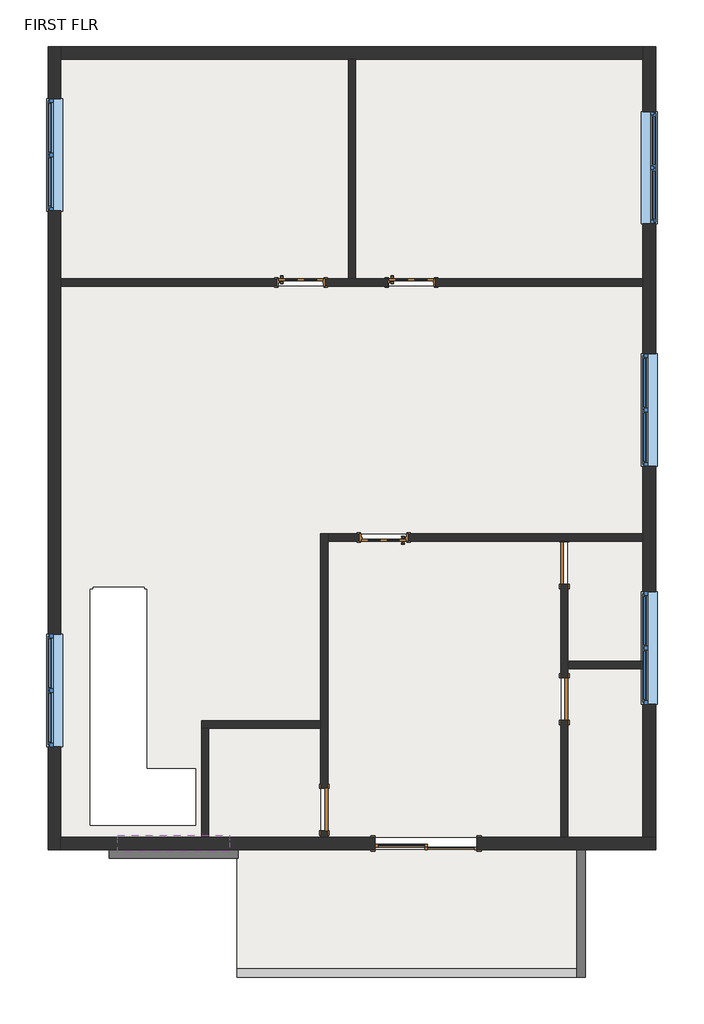
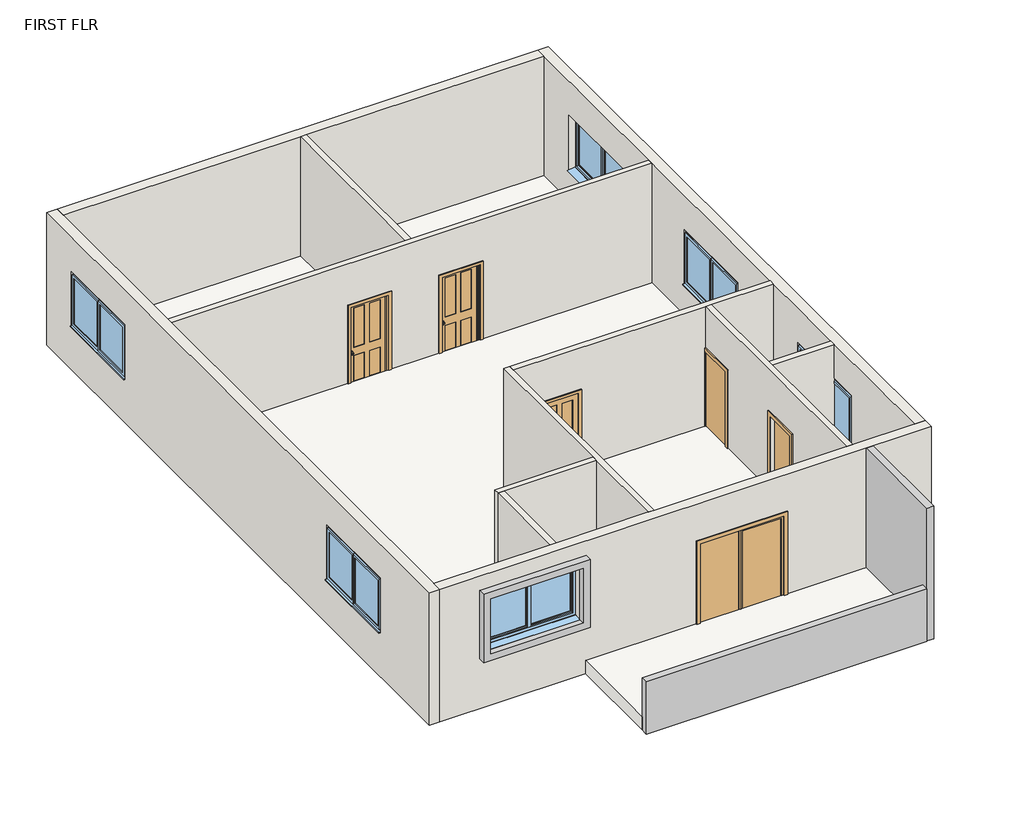
# One storey, incomplete: 12 walls, 7 doors, 6 windows, 3 proxies, 1 slab.
"""IFC4 building model written with IfcOpenShell, lengths in millimetres."""

from ifc_helpers import new_model, si_unit, frame, origin, place, context, project, spatial, polyline, outline, extrude, faceted_brep, transform, mapped, element, save
from components import generic_models_1_generic_models_1_b00c282c, generic_models_2_generic_models_2_90455f6d, generic_models_6_generic_models_6_ad273a16, door_d4d75d1e, door_interior_single_4_panel_wood_door_interior_single_4_d89ef9d3, door_1fe7f57d, door_e00f436c, w2_w2_7b90d420

model = new_model("IFC4")

# Units and contexts
model_context = context("Model", 3, world=origin())
ifc_project = project(units=[si_unit("LENGTHUNIT", "METRE", prefix="MILLI")], contexts=[model_context])

# Site, building, storey
site = spatial("IfcSite", under=ifc_project)
building = spatial("IfcBuilding", under=site)
storey = spatial("IfcBuildingStorey", under=building, Name="FIRST FLR", Elevation=3352.8)

# Proxies
placement = place(None, origin())
generic_models_1_generic_models_1_shape = generic_models_1_generic_models_1_b00c282c(model_context)
element("IfcBuildingElementProxy", 1, Name="Generic Models 1 : Generic Models 1", ObjectType="Generic Models 1 : Generic Models 1", at=placement, inside=storey, context=model_context, shape_type="MappedRepresentation", body=[
    mapped(generic_models_1_generic_models_1_shape, transform((0.0, 0.0, 0.0), x_axis=(1.0, 0.0, 0.0), y_axis=(0.0, 1.0, 0.0), z_axis=(0.0, 0.0, 1.0))),
])
generic_models_2_generic_models_2_shape = generic_models_2_generic_models_2_90455f6d(model_context)
element("IfcBuildingElementProxy", 2, Name="Generic Models 2 : Generic Models 2", ObjectType="Generic Models 2 : Generic Models 2", at=placement, inside=storey, context=model_context, shape_type="MappedRepresentation", body=[
    mapped(generic_models_2_generic_models_2_shape, transform((0.0, 0.0, 0.0), x_axis=(1.0, 0.0, 0.0), y_axis=(0.0, 1.0, 0.0), z_axis=(0.0, 0.0, 1.0))),
])
generic_models_6_generic_models_6_shape = generic_models_6_generic_models_6_ad273a16(model_context)
element("IfcBuildingElementProxy", 3, Name="Generic Models 6 : Generic Models 6", ObjectType="Generic Models 6 : Generic Models 6", at=placement, inside=storey, context=model_context, shape_type="MappedRepresentation", body=[
    mapped(generic_models_6_generic_models_6_shape, transform((0.0, 0.0, 0.0), x_axis=(1.0, 0.0, 0.0), y_axis=(0.0, 1.0, 0.0), z_axis=(0.0, 0.0, 1.0))),
])

# Doors
door_shape = door_d4d75d1e(model_context)
element("IfcDoor", 4, ObjectType="Door-Double-Sliding : 72\" x 84\"", at=placement, inside=storey, context=model_context, shape_type="MappedRepresentation", body=[
    mapped(door_shape, transform((24.4764037, -4030.9938352, 3352.8), x_axis=(-1.0, 0.0, 0.0), y_axis=(0.0, -1.0, 0.0), z_axis=(0.0, 0.0, 1.0))),
])
door_interior_single_4_panel_wood_door_interior_single_4_shape = door_interior_single_4_panel_wood_door_interior_single_4_d89ef9d3(model_context)
element("IfcDoor", 5, ObjectType="Door-Interior-Single-4_Panel-Wood : Door-Interior-Single-4_Panel-Wood", at=placement, inside=storey, context=model_context, shape_type="MappedRepresentation", body=[
    mapped(door_interior_single_4_panel_wood_door_interior_single_4_shape, transform((-241.5474631, 5903.5811648, 3352.8), x_axis=(1.0, 0.0, 0.0), y_axis=(0.0, 1.0, 0.0), z_axis=(0.0, 0.0, 1.0))),
])
element("IfcDoor", 6, ObjectType="Door-Interior-Single-4_Panel-Wood : Door-Interior-Single-4_Panel-Wood", at=placement, inside=storey, context=model_context, shape_type="MappedRepresentation", body=[
    mapped(door_interior_single_4_panel_wood_door_interior_single_4_shape, transform((-2222.7474631, 5903.5811648, 3352.8), x_axis=(1.0, 0.0, 0.0), y_axis=(0.0, 1.0, 0.0), z_axis=(0.0, 0.0, 1.0))),
])
element("IfcDoor", 7, ObjectType="Door-Interior-Single-4_Panel-Wood : Door-Interior-Single-4_Panel-Wood", at=placement, inside=storey, context=model_context, shape_type="MappedRepresentation", body=[
    mapped(door_interior_single_4_panel_wood_door_interior_single_4_shape, transform((-737.5235963, 1325.2311648, 3352.8), x_axis=(-1.0, 0.0, 0.0), y_axis=(0.0, -1.0, 0.0), z_axis=(0.0, 0.0, 1.0))),
])
door_2_shape = door_1fe7f57d(model_context)
element("IfcDoor", 8, ObjectType="Single-Flush : 30\" x 80\"", at=placement, inside=storey, context=model_context, shape_type="MappedRepresentation", body=[
    mapped(door_2_shape, transform((2501.6525369, 871.2061648, 3352.8), x_axis=(0.0, 1.0, 0.0), y_axis=(-1.0, 0.0, 0.0), z_axis=(0.0, 0.0, 1.0))),
])
element("IfcDoor", 9, ObjectType="Single-Flush : 30\" x 80\"", at=placement, inside=storey, context=model_context, shape_type="MappedRepresentation", body=[
    mapped(door_2_shape, transform((2501.6525369, -1567.1938352, 3352.8), x_axis=(0.0, -1.0, 0.0), y_axis=(1.0, 0.0, 0.0), z_axis=(0.0, 0.0, 1.0))),
])
door_3_shape = door_e00f436c(model_context)
element("IfcDoor", 10, ObjectType="Single-Flush : 30\" x 80\"", at=placement, inside=storey, context=model_context, shape_type="MappedRepresentation", body=[
    mapped(door_3_shape, transform((-1804.3235963, -3548.3938352, 3352.8), x_axis=(0.0, 1.0, 0.0), y_axis=(-1.0, 0.0, 0.0), z_axis=(0.0, 0.0, 1.0))),
])

# Slab
element("IfcSlab", 11, ObjectType="MARBLE FLOORING 1'", at=placement, inside=storey, context=model_context, shape_type="SweptSolid", body=[
    extrude(outline(polyline([(-1371.8474631, 9900.9061648), (-1371.8474631, 5963.9061648), (-6528.0474631, 5963.9061648), (-6528.0474631, 9900.9061648), (-1371.8474631, 9900.9061648)])), frame((0.0, 0.0, 3352.8), z_axis=(0.0, 0.0, 1.0), x_axis=(1.0, 0.0, 0.0)), (0.0, 0.0, 1.0), 304.8),
    extrude(outline(polyline([(3911.3525369, 9900.9061648), (3911.3525369, 5963.9061648), (-1244.8474631, 5963.9061648), (-1244.8474631, 9900.9061648), (3911.3525369, 9900.9061648)])), frame((0.0, 0.0, 3352.8), z_axis=(0.0, 0.0, 1.0), x_axis=(1.0, 0.0, 0.0)), (0.0, 0.0, 1.0), 304.8),
    extrude(outline(polyline([(-1867.8235963, -2087.8938352), (-1867.8235963, -4043.6938352), (-3874.4235963, -4043.6938352), (-3874.4235963, -2087.8938352), (-1867.8235963, -2087.8938352)])), frame((0.0, 0.0, 3352.8), z_axis=(0.0, 0.0, 1.0), x_axis=(1.0, 0.0, 0.0)), (0.0, 0.0, 1.0), 304.8),
    extrude(outline(polyline([(3911.3525369, 1264.9061648), (3911.3525369, -894.0938352), (2565.1525369, -894.0938352), (2565.1525369, 1264.9061648), (3911.3525369, 1264.9061648)])), frame((0.0, 0.0, 3352.8), z_axis=(0.0, 0.0, 1.0), x_axis=(1.0, 0.0, 0.0)), (0.0, 0.0, 1.0), 304.8),
    extrude(outline(polyline([(3912.9151699, -1021.0938352), (3912.9151699, -4043.6938352), (2565.1525369, -4043.6938352), (2565.1525369, -1021.0938352), (3912.9151699, -1021.0938352)])), frame((0.0, 0.0, 3352.8), z_axis=(0.0, 0.0, 1.0), x_axis=(1.0, 0.0, 0.0)), (0.0, 0.0, 1.0), 304.8),
    extrude(outline(polyline([(2438.1525369, 1264.9061648), (2438.1525369, -4043.6938352), (-1740.8235963, -4043.6938352), (-1740.8235963, 1264.9061648), (2438.1525369, 1264.9061648)])), frame((0.0, 0.0, 3352.8), z_axis=(0.0, 0.0, 1.0), x_axis=(1.0, 0.0, 0.0)), (0.0, 0.0, 1.0), 304.8),
    extrude(outline(polyline([(-4001.4235963, -4043.6938352), (-6528.0474631, -4043.6938352), (-6528.0474631, 5836.9061648), (3911.3525369, 5836.9061648), (3911.3525369, 1391.9061648), (-1867.8235963, 1391.9061648), (-1867.8235963, -1960.8938352), (-4001.4235963, -1960.8938352), (-4001.4235963, -4043.6938352)]), holes=[polyline([(-4986.3750936, -2818.257314), (-4986.3750936, 402.8727516), (-5037.1750936, 402.8727516), (-5037.1750936, 434.6227516), (-5951.5750936, 434.6227516), (-5951.5750936, 402.8727516), (-6002.3750936, 402.8727516), (-6002.3750936, -3834.257314), (-4109.8601025, -3834.257314), (-4109.8601025, -2818.257314), (-4986.3750936, -2818.257314)])]), frame((0.0, 0.0, 3352.8), z_axis=(0.0, 0.0, 1.0), x_axis=(1.0, 0.0, 0.0)), (0.0, 0.0, 1.0), 304.8),
    extrude(outline(polyline([(2729.4546869, -4272.2938352), (2729.4546869, -6405.8938352), (-3366.5453131, -6405.8938352), (-3366.5453131, -4272.2938352), (2729.4546869, -4272.2938352)])), frame((0.0, 0.0, 3352.8), z_axis=(0.0, 0.0, 1.0), x_axis=(1.0, 0.0, 0.0)), (0.0, 0.0, 1.0), 304.8),
])

# Walls
element("IfcWall", 12, ObjectType="EXTERIOR WALL 9\"", at=placement, inside=storey, context=model_context, shape_type="Brep", body=[
    faceted_brep([(-6756.6474631, 10129.5061648, 3352.8), (-6756.6474631, -4272.2938352, 3352.8), (-6756.6474631, -4272.2938352, 6400.8), (-6756.6474631, 10129.5061648, 6400.8), (-6756.6474631, -409.7938352, 4352.8), (-6756.6474631, -409.7938352, 5612.8), (-6756.6474631, -2419.7938352, 5612.8), (-6756.6474631, -2419.7938352, 4352.8), (-6756.6474631, 9191.4061648, 4352.8), (-6756.6474631, 9191.4061648, 5612.8), (-6756.6474631, 7181.4061648, 5612.8), (-6756.6474631, 7181.4061648, 4352.8), (-6528.0474631, 10129.5061648, 3352.8), (-6528.0474631, 10129.5061648, 6400.8), (-6528.0474631, 9900.9061648, 6400.8), (-6528.0474631, 5963.9061648, 6400.8), (-6528.0474631, 5836.9061648, 6400.8), (-6528.0474631, -4043.6938352, 6400.8), (-6528.0474631, -4272.2938352, 6400.8), (-6528.0474631, -4272.2938352, 3352.8), (-6528.0474631, -4043.6938352, 3352.8), (-6528.0474631, 5836.9061648, 3352.8), (-6528.0474631, 5963.9061648, 3352.8), (-6528.0474631, 9900.9061648, 3352.8), (-6528.0474631, -409.7938352, 4352.8), (-6528.0474631, -2419.7938352, 4352.8), (-6528.0474631, -2419.7938352, 5612.8), (-6528.0474631, -409.7938352, 5612.8), (-6528.0474631, 9191.4061648, 4352.8), (-6528.0474631, 7181.4061648, 4352.8), (-6528.0474631, 7181.4061648, 5612.8), (-6528.0474631, 9191.4061648, 5612.8)], [[[0, 1, 2, 3], [4, 5, 6, 7], [8, 9, 10, 11]], [[12, 13, 14, 15, 16, 17, 18, 19, 20, 21, 22, 23], [24, 25, 26, 27], [28, 29, 30, 31]], [[1, 0, 12, 23, 22, 21, 20, 19]], [[3, 2, 18, 17, 16, 15, 14, 13]], [[2, 1, 19, 18]], [[0, 3, 13, 12]], [[5, 4, 24, 27]], [[6, 5, 27, 26]], [[7, 6, 26, 25]], [[4, 7, 25, 24]], [[9, 8, 28, 31]], [[10, 9, 31, 30]], [[11, 10, 30, 29]], [[8, 11, 29, 28]]]),
])
element("IfcWall", 13, ObjectType="EXTERIOR WALL 9\"", at=placement, inside=storey, context=model_context, shape_type="Brep", body=[
    faceted_brep([(-6528.0474631, -4272.2938352, 3352.8), (-889.9235963, -4272.2938352, 3352.8), (-889.9235963, -4272.2938352, 5486.4), (938.8764037, -4272.2938352, 5486.4), (938.8764037, -4272.2938352, 3352.8), (4139.9525369, -4272.2938352, 3352.8), (4139.9525369, -4272.2938352, 6400.8), (-6528.0474631, -4272.2938352, 6400.8), (-3503.7474631, -4272.2938352, 4657.6), (-5513.7474631, -4272.2938352, 4657.6), (-5513.7474631, -4272.2938352, 5917.6), (-3503.7474631, -4272.2938352, 5917.6), (-889.9235963, -4043.6938352, 5486.4), (-889.9235963, -4043.6938352, 3352.8), (-1740.8235963, -4043.6938352, 3352.8), (-1867.8235963, -4043.6938352, 3352.8), (-3874.4235963, -4043.6938352, 3352.8), (-4001.4235963, -4043.6938352, 3352.8), (-6528.0474631, -4043.6938352, 3352.8), (-6528.0474631, -4043.6938352, 6400.8), (-4001.4235963, -4043.6938352, 6400.8), (-3874.4235963, -4043.6938352, 6400.8), (-1867.8235963, -4043.6938352, 6400.8), (-1740.8235963, -4043.6938352, 6400.8), (2438.1525369, -4043.6938352, 6400.8), (2565.1525369, -4043.6938352, 6400.8), (3911.3525369, -4043.6938352, 6400.8), (4139.9525369, -4043.6938352, 6400.8), (4139.9525369, -4043.6938352, 3352.8), (3911.3525369, -4043.6938352, 3352.8), (2565.1525369, -4043.6938352, 3352.8), (2438.1525369, -4043.6938352, 3352.8), (938.8764037, -4043.6938352, 3352.8), (938.8764037, -4043.6938352, 5486.4), (-3503.7474631, -4043.6938352, 4657.6), (-3503.7474631, -4043.6938352, 5917.6), (-5513.7474631, -4043.6938352, 5917.6), (-5513.7474631, -4043.6938352, 4657.6)], [[[0, 1, 2, 3, 4, 5, 6, 7], [8, 9, 10, 11]], [[12, 13, 14, 15, 16, 17, 18, 19, 20, 21, 22, 23, 24, 25, 26, 27, 28, 29, 30, 31, 32, 33], [34, 35, 36, 37]], [[18, 17, 16, 15, 14, 13, 1, 0]], [[32, 31, 30, 29, 28, 5, 4]], [[7, 6, 27, 26, 25, 24, 23, 22, 21, 20, 19]], [[0, 7, 19, 18]], [[6, 5, 28, 27]], [[35, 34, 8, 11]], [[36, 35, 11, 10]], [[37, 36, 10, 9]], [[34, 37, 9, 8]], [[4, 3, 33, 32]], [[2, 1, 13, 12]], [[3, 2, 12, 33]]]),
])
element("IfcWall", 14, ObjectType="EXTERIOR WALL 9\"", at=placement, inside=storey, context=model_context, shape_type="Brep", body=[
    faceted_brep([(4139.9525369, -4043.6938352, 3352.8), (4139.9525369, 10129.5061648, 3352.8), (4139.9525369, 10129.5061648, 6400.8), (4139.9525369, -4043.6938352, 6400.8), (4139.9525369, 4619.4061648, 4352.8), (4139.9525369, 2609.4061648, 4352.8), (4139.9525369, 2609.4061648, 5612.8), (4139.9525369, 4619.4061648, 5612.8), (4139.9525369, 352.2061648, 4352.8), (4139.9525369, -1657.7938352, 4352.8), (4139.9525369, -1657.7938352, 5612.8), (4139.9525369, 352.2061648, 5612.8), (4139.9525369, 6952.8061648, 4352.8), (4139.9525369, 6952.8061648, 5612.8), (4139.9525369, 8962.8061648, 5612.8), (4139.9525369, 8962.8061648, 4352.8), (3911.3525369, -4043.6938352, 3352.8), (3911.3525369, -4043.6938352, 6400.8), (3911.3525369, -1021.0938352, 6400.8), (3911.3525369, -894.0938352, 6400.8), (3911.3525369, 5836.9061648, 6400.8), (3911.3525369, 5963.9061648, 6400.8), (3911.3525369, 9900.9061648, 6400.8), (3911.3525369, 10129.5061648, 6400.8), (3911.3525369, 10129.5061648, 3352.8), (3911.3525369, 9900.9061648, 3352.8), (3911.3525369, 5963.9061648, 3352.8), (3911.3525369, 5836.9061648, 3352.8), (3911.3525369, -894.0938352, 3352.8), (3911.3525369, -1021.0938352, 3352.8), (3911.3525369, 4619.4061648, 4352.8), (3911.3525369, 4619.4061648, 5612.8), (3911.3525369, 2609.4061648, 5612.8), (3911.3525369, 2609.4061648, 4352.8), (3911.3525369, 352.2061648, 4352.8), (3911.3525369, 352.2061648, 5612.8), (3911.3525369, -1657.7938352, 5612.8), (3911.3525369, -1657.7938352, 4352.8), (3911.3525369, 6952.8061648, 4352.8), (3911.3525369, 8962.8061648, 4352.8), (3911.3525369, 8962.8061648, 5612.8), (3911.3525369, 6952.8061648, 5612.8)], [[[0, 1, 2, 3], [4, 5, 6, 7], [8, 9, 10, 11], [12, 13, 14, 15]], [[16, 17, 18, 19, 20, 21, 22, 23, 24, 25, 26, 27, 28, 29], [30, 31, 32, 33], [34, 35, 36, 37], [38, 39, 40, 41]], [[1, 0, 16, 29, 28, 27, 26, 25, 24]], [[3, 2, 23, 22, 21, 20, 19, 18, 17]], [[0, 3, 17, 16]], [[2, 1, 24, 23]], [[31, 30, 4, 7]], [[32, 31, 7, 6]], [[33, 32, 6, 5]], [[30, 33, 5, 4]], [[35, 34, 8, 11]], [[36, 35, 11, 10]], [[37, 36, 10, 9]], [[34, 37, 9, 8]], [[13, 12, 38, 41]], [[14, 13, 41, 40]], [[15, 14, 40, 39]], [[12, 15, 39, 38]]]),
])
element("IfcWall", 15, ObjectType="EXTERIOR WALL 9\"", at=placement, inside=storey, context=model_context, shape_type="Brep", body=[
    faceted_brep([(3911.3525369, 10129.5061648, 3352.8), (-6528.0474631, 10129.5061648, 3352.8), (-6528.0474631, 10129.5061648, 6400.8), (3911.3525369, 10129.5061648, 6400.8), (3911.3525369, 9900.9061648, 3352.8), (3911.3525369, 9900.9061648, 6400.8), (-1244.8474631, 9900.9061648, 6400.8), (-1371.8474631, 9900.9061648, 6400.8), (-6528.0474631, 9900.9061648, 6400.8), (-6528.0474631, 9900.9061648, 3352.8), (-1371.8474631, 9900.9061648, 3352.8), (-1244.8474631, 9900.9061648, 3352.8)], [[[0, 1, 2, 3]], [[4, 5, 6, 7, 8, 9, 10, 11]], [[1, 0, 4, 11, 10, 9]], [[3, 2, 8, 7, 6, 5]], [[0, 3, 5, 4]], [[2, 1, 9, 8]]]),
])
element("IfcWall", 16, ObjectType="INTERIOR WALL 5\"", at=placement, inside=storey, context=model_context, shape_type="SweptSolid", body=[
    extrude(outline(polyline([(-1371.8474631, 5963.9061648), (-1371.8474631, 9900.9061648), (-1244.8474631, 9900.9061648), (-1244.8474631, 5963.9061648), (-1371.8474631, 5963.9061648)])), frame((0.0, 0.0, 3352.8), z_axis=(0.0, 0.0, 1.0), x_axis=(1.0, 0.0, 0.0)), (0.0, 0.0, 1.0), 3048.0),
])
element("IfcWall", 17, ObjectType="INTERIOR WALL 5\"", at=placement, inside=storey, context=model_context, shape_type="Brep", body=[
    faceted_brep([(3911.3525369, 5836.9061648, 6400.8), (-6528.0474631, 5836.9061648, 6400.8), (-6528.0474631, 5836.9061648, 3352.8), (-2654.5474631, 5836.9061648, 3352.8), (-2654.5474631, 5836.9061648, 5410.2), (-1790.9474631, 5836.9061648, 5410.2), (-1790.9474631, 5836.9061648, 3352.8), (-673.3474631, 5836.9061648, 3352.8), (-673.3474631, 5836.9061648, 5410.2), (190.2525369, 5836.9061648, 5410.2), (190.2525369, 5836.9061648, 3352.8), (3911.3525369, 5836.9061648, 3352.8), (-6528.0474631, 5963.9061648, 6400.8), (-1371.8474631, 5963.9061648, 6400.8), (-1244.8474631, 5963.9061648, 6400.8), (3911.3525369, 5963.9061648, 6400.8), (3911.3525369, 5963.9061648, 3352.8), (190.2525369, 5963.9061648, 3352.8), (190.2525369, 5963.9061648, 5410.2), (-673.3474631, 5963.9061648, 5410.2), (-673.3474631, 5963.9061648, 3352.8), (-1244.8474631, 5963.9061648, 3352.8), (-1371.8474631, 5963.9061648, 3352.8), (-1790.9474631, 5963.9061648, 3352.8), (-1790.9474631, 5963.9061648, 5410.2), (-2654.5474631, 5963.9061648, 5410.2), (-2654.5474631, 5963.9061648, 3352.8), (-6528.0474631, 5963.9061648, 3352.8)], [[[0, 1, 2, 3, 4, 5, 6, 7, 8, 9, 10, 11]], [[12, 13, 14, 15, 16, 17, 18, 19, 20, 21, 22, 23, 24, 25, 26, 27]], [[16, 11, 10, 17]], [[2, 27, 26, 3]], [[20, 7, 6, 23, 22, 21]], [[1, 0, 15, 14, 13, 12]], [[0, 11, 16, 15]], [[2, 1, 12, 27]], [[9, 18, 17, 10]], [[18, 9, 8, 19]], [[19, 8, 7, 20]], [[5, 24, 23, 6]], [[24, 5, 4, 25]], [[25, 4, 3, 26]]]),
])
element("IfcWall", 18, ObjectType="INTERIOR WALL 5\"", at=placement, inside=storey, context=model_context, shape_type="Brep", body=[
    faceted_brep([(-1867.8235963, 1391.9061648, 3352.8), (-1867.8235963, -1960.8938352, 3352.8), (-1867.8235963, -2087.8938352, 3352.8), (-1867.8235963, -3167.3938352, 3352.8), (-1867.8235963, -3167.3938352, 5384.8), (-1867.8235963, -3929.3938352, 5384.8), (-1867.8235963, -3929.3938352, 3352.8), (-1867.8235963, -4043.6938352, 3352.8), (-1867.8235963, -4043.6938352, 6400.8), (-1867.8235963, -2087.8938352, 6400.8), (-1867.8235963, -1960.8938352, 6400.8), (-1867.8235963, 1391.9061648, 6400.8), (-1740.8235963, -3167.3938352, 5384.8), (-1740.8235963, -3167.3938352, 3352.8), (-1740.8235963, 1264.9061648, 3352.8), (-1740.8235963, 1391.9061648, 3352.8), (-1740.8235963, 1391.9061648, 6400.8), (-1740.8235963, 1264.9061648, 6400.8), (-1740.8235963, -4043.6938352, 6400.8), (-1740.8235963, -4043.6938352, 3352.8), (-1740.8235963, -3929.3938352, 3352.8), (-1740.8235963, -3929.3938352, 5384.8)], [[[0, 1, 2, 3, 4, 5, 6, 7, 8, 9, 10, 11]], [[12, 13, 14, 15, 16, 17, 18, 19, 20, 21]], [[20, 19, 7, 6]], [[15, 14, 13, 3, 2, 1, 0]], [[11, 10, 9, 8, 18, 17, 16]], [[8, 7, 19, 18]], [[0, 11, 16, 15]], [[4, 3, 13, 12]], [[5, 4, 12, 21]], [[6, 5, 21, 20]]]),
])
element("IfcWall", 19, ObjectType="INTERIOR WALL 5\"", at=placement, inside=storey, context=model_context, shape_type="Brep", body=[
    faceted_brep([(-4001.4235963, -2087.8938352, 3352.8), (-3874.4235963, -2087.8938352, 3352.8), (-1867.8235963, -2087.8938352, 3352.8), (-1867.8235963, -2087.8938352, 6400.8), (-3874.4235963, -2087.8938352, 6400.8), (-4001.4235963, -2087.8938352, 6400.8), (-4001.4235963, -1960.8938352, 3352.8), (-4001.4235963, -1960.8938352, 6400.8), (-1867.8235963, -1960.8938352, 6400.8), (-1867.8235963, -1960.8938352, 3352.8)], [[[0, 1, 2, 3, 4, 5]], [[6, 7, 8, 9]], [[2, 1, 0, 6, 9]], [[5, 4, 3, 8, 7]], [[0, 5, 7, 6]], [[3, 2, 9, 8]]]),
])
element("IfcWall", 20, ObjectType="INTERIOR WALL 5\"", at=placement, inside=storey, context=model_context, shape_type="SweptSolid", body=[
    extrude(outline(polyline([(-3874.4235963, -2087.8938352), (-3874.4235963, -4043.6938352), (-4001.4235963, -4043.6938352), (-4001.4235963, -2087.8938352), (-3874.4235963, -2087.8938352)])), frame((0.0, 0.0, 3352.8), z_axis=(0.0, 0.0, 1.0), x_axis=(1.0, 0.0, 0.0)), (0.0, 0.0, 1.0), 3048.0),
])
element("IfcWall", 21, ObjectType="INTERIOR WALL 5\"", at=placement, inside=storey, context=model_context, shape_type="Brep", body=[
    faceted_brep([(3910.6764037, 1264.9061648, 3352.8), (3910.6764037, 1264.9061648, 6400.8), (2565.1525369, 1264.9061648, 6400.8), (2438.1525369, 1264.9061648, 6400.8), (-1740.8235963, 1264.9061648, 6400.8), (-1740.8235963, 1264.9061648, 3352.8), (-1169.3235963, 1264.9061648, 3352.8), (-1169.3235963, 1264.9061648, 5410.2), (-305.7235963, 1264.9061648, 5410.2), (-305.7235963, 1264.9061648, 3352.8), (2438.1525369, 1264.9061648, 3352.8), (2565.1525369, 1264.9061648, 3352.8), (3910.6764037, 1391.9061648, 6400.8), (3910.6764037, 1391.9061648, 3352.8), (-305.7235963, 1391.9061648, 3352.8), (-305.7235963, 1391.9061648, 5410.2), (-1169.3235963, 1391.9061648, 5410.2), (-1169.3235963, 1391.9061648, 3352.8), (-1740.8235963, 1391.9061648, 3352.8), (-1740.8235963, 1391.9061648, 6400.8)], [[[0, 1, 2, 3, 4, 5, 6, 7, 8, 9, 10, 11]], [[12, 13, 14, 15, 16, 17, 18, 19]], [[13, 0, 11, 10, 9, 14]], [[5, 18, 17, 6]], [[1, 0, 13, 12]], [[4, 3, 2, 1, 12, 19]], [[5, 4, 19, 18]], [[16, 7, 6, 17]], [[7, 16, 15, 8]], [[8, 15, 14, 9]]]),
])
element("IfcWall", 22, ObjectType="INTERIOR WALL 5\"", at=placement, inside=storey, context=model_context, shape_type="Brep", body=[
    faceted_brep([(2438.1525369, -1948.1938352, 5384.8), (2438.1525369, -1948.1938352, 3352.8), (2438.1525369, -4043.6938352, 3352.8), (2438.1525369, -4043.6938352, 6400.8), (2438.1525369, 1264.9061648, 6400.8), (2438.1525369, 1264.9061648, 3352.8), (2438.1525369, 1252.2061648, 3352.8), (2438.1525369, 1252.2061648, 5384.8), (2438.1525369, 490.2061648, 5384.8), (2438.1525369, 490.2061648, 3352.8), (2438.1525369, -1186.1938352, 3352.8), (2438.1525369, -1186.1938352, 5384.8), (2565.1525369, -4043.6938352, 3352.8), (2565.1525369, -1948.1938352, 3352.8), (2565.1525369, -1948.1938352, 5384.8), (2565.1525369, -1186.1938352, 5384.8), (2565.1525369, -1186.1938352, 3352.8), (2565.1525369, -1021.0938352, 3352.8), (2565.1525369, -894.0938352, 3352.8), (2565.1525369, 490.2061648, 3352.8), (2565.1525369, 490.2061648, 5384.8), (2565.1525369, 1252.2061648, 5384.8), (2565.1525369, 1252.2061648, 3352.8), (2565.1525369, 1264.9061648, 3352.8), (2565.1525369, 1264.9061648, 6400.8), (2565.1525369, -894.0938352, 6400.8), (2565.1525369, -1021.0938352, 6400.8), (2565.1525369, -4043.6938352, 6400.8)], [[[0, 1, 2, 3, 4, 5, 6, 7, 8, 9, 10, 11]], [[12, 13, 14, 15, 16, 17, 18, 19, 20, 21, 22, 23, 24, 25, 26, 27]], [[23, 22, 6, 5]], [[10, 9, 19, 18, 17, 16]], [[2, 1, 13, 12]], [[4, 3, 27, 26, 25, 24]], [[3, 2, 12, 27]], [[5, 4, 24, 23]], [[7, 6, 22, 21]], [[8, 7, 21, 20]], [[9, 8, 20, 19]], [[14, 13, 1, 0]], [[15, 14, 0, 11]], [[16, 15, 11, 10]]]),
])
element("IfcWall", 23, ObjectType="INTERIOR WALL 5\"", at=placement, inside=storey, context=model_context, shape_type="SweptSolid", body=[
    extrude(outline(polyline([(3911.3525369, -1021.0938352), (2565.1525369, -1021.0938352), (2565.1525369, -894.0938352), (3911.3525369, -894.0938352), (3911.3525369, -1021.0938352)])), frame((0.0, 0.0, 3352.8), z_axis=(0.0, 0.0, 1.0), x_axis=(1.0, 0.0, 0.0)), (0.0, 0.0, 1.0), 3048.0),
])

# Windows
w2_w2_shape = w2_w2_7b90d420(model_context)
element("IfcWindow", 24, ObjectType="w2 : w2", at=placement, inside=storey, context=model_context, shape_type="MappedRepresentation", body=[
    mapped(w2_w2_shape, transform((4025.6525369, -652.7938352, 3352.8), x_axis=(0.0, -1.0, 0.0), y_axis=(1.0, 0.0, 0.0), z_axis=(0.0, 0.0, 1.0))),
])
element("IfcWindow", 25, ObjectType="w2 : w2", at=placement, inside=storey, context=model_context, shape_type="MappedRepresentation", body=[
    mapped(w2_w2_shape, transform((4025.6525369, 3614.4061648, 3352.8), x_axis=(0.0, -1.0, 0.0), y_axis=(1.0, 0.0, 0.0), z_axis=(0.0, 0.0, 1.0))),
])
element("IfcWindow", 26, ObjectType="w2 : w2", at=placement, inside=storey, context=model_context, shape_type="MappedRepresentation", body=[
    mapped(w2_w2_shape, transform((-6642.3474631, -1414.7938352, 3352.8), x_axis=(0.0, -1.0, 0.0), y_axis=(1.0, 0.0, 0.0), z_axis=(0.0, 0.0, 1.0))),
])
element("IfcWindow", 27, ObjectType="w2 : w2", at=placement, inside=storey, context=model_context, shape_type="MappedRepresentation", body=[
    mapped(w2_w2_shape, transform((-4508.7474631, -4157.9938352, 3657.6), x_axis=(-1.0, 0.0, 0.0), y_axis=(0.0, -1.0, 0.0), z_axis=(0.0, 0.0, 1.0))),
])
element("IfcWindow", 28, ObjectType="w2 : w2", at=placement, inside=storey, context=model_context, shape_type="MappedRepresentation", body=[
    mapped(w2_w2_shape, transform((4025.6525369, 7957.8061648, 3352.8), x_axis=(0.0, 1.0, 0.0), y_axis=(-1.0, 0.0, 0.0), z_axis=(0.0, 0.0, 1.0))),
])
element("IfcWindow", 29, ObjectType="w2 : w2", at=placement, inside=storey, context=model_context, shape_type="MappedRepresentation", body=[
    mapped(w2_w2_shape, transform((-6642.3474631, 8186.4061648, 3352.8), x_axis=(0.0, -1.0, 0.0), y_axis=(1.0, 0.0, 0.0), z_axis=(0.0, 0.0, 1.0))),
])

save(model, "model.ifc")

# Revit data of these elements
# Type "Door-Double-Sliding : 72\" x 84\""
#   Type Mark = "8"
#   Construction Type Id = "opn-d45"
#   Assembly Code = "C1020"
#   Analytic Construction = "Wood frame, double glass door "
#   Thickness = 0' - 2"
#   Thermal Resistance (R) = 1.8150 (h·ft²·°F)/BTU
#   Heat Transfer Coefficient (U) = 0.5510 BTU/(h·ft²·°F)
#   Height = 7' - 0"
#   Rail Width = 0' - 2"
#   Stiles = 0' - 2"
#   Trim Projection Ext = 0' - 1"
#   Trim Projection Int = 0' - 1"
#   Trim Width = 0' - 3"
#   Width = 6' - 0"
#   Define Thermal Properties by = 1
#   Glazing = Glass
#   Panel Material = Wood - Birch - Solid Stained Light Low Gloss
#   Trim Material = Paint - Sienna
#   Visual Light Transmittance = 0
#   Solar Heat Gain Coefficient = 0
#   Function = (empty or 0)
#   Wall Closure = (empty or 0)
# Type "Door-Interior-Single-4_Panel-Wood : Door-Interior-Single-4_Panel-Wood"
#   Type Mark = "9"
#   Assembly Code = "C1020300"
#   Analytic Construction = "Wooden"
#   Top Rail = 0' - 4 11/16"
#   Thickness = 0' - 1 3/8"
#   Thermal Resistance (R) = 2.5876 (h·ft²·°F)/BTU
#   Swing Angle [instance default] = 90.00°
#   Stiles = 0' - 4 3/4"
#   Rough Width = 2' - 10"
#   Rough Height = 6' - 9"
#   Mullion = 0' - 4 1/2"
#   Lock Rail = 0' - 7 1/2"
#   Height = 6' - 8"
#   Width = 2' - 8"
#   Heat Transfer Coefficient (U) = 0.3865 BTU/(h·ft²·°F)
#   Bottom Rail = 0' - 9 1/8"
#   Trim Material = Cherry
#   Panel Material = Cherry
#   Frame Material = Cherry
#   Door Handle Material = Aluminum
#   Visual Light Transmittance = 0
#   Solar Heat Gain Coefficient = 0
#   Wall Closure = (empty or 0)
#   Function = (empty or 0)
# Type "Single-Flush : 30\" x 80\""
#   Type Mark = "5"
#   Construction Type Id = "MDOOR"
#   Assembly Code = "C1020"
#   Analytic Construction = "Metal"
#   Thickness = 0' - 2"
#   Heat Transfer Coefficient (U) = 0.651978 BTU/(h·ft²·°F)
#   Height = 6' - 8"
#   Trim Projection Ext = 0' - 1"
#   Trim Projection Int = 0' - 1"
#   Trim Width = 0' - 3"
#   Width = 2' - 6"
#   Define Thermal Properties by = 1
#   Define Thermal Properties by = 1
#   Door Material = Door - Panel
#   Frame Material = Door - Frame
#   Visual Light Transmittance = 0
#   Solar Heat Gain Coefficient = 0
#   Function = (empty or 0)
#   Wall Closure = (empty or 0)
# Type "MARBLE FLOORING 1'"
#   Assembly Code = "B1010"
#   Function = 0
#   Layers, outside or top first: 1' - 0" "MARBLE MATERIAL" (function 1)
# Type "EXTERIOR WALL 9\""
#   Assembly Code = "B2010"
#   Layers, outside or top first: 0' - 9" "OFF WHITE COLOUR" (function 1)
# Type "INTERIOR WALL 5\""
#   Assembly Code = "B2010"
#   Layers, outside or top first: 0' - 5" "OFF WHITE COLOUR" (function 1)
# Type "w2 : w2"
#   Type Mark = "18"
#   Operation = "DoublePanelVertical"
#   Keynote = "16.05.01"
#   Analytic Construction = "<None>"
#   Rough Width = 6' - 7.13386"
#   Rough Height = 4' - 1.6063"
#   Rahmentiefe = 0' - 2.3622"
#   Rahmenhöhe unten = 0' - 3.14961"
#   Rahmehöhe oben = 0' - 3.14961"
#   Rahmenbreite = 0' - 2.3622"
#   Heat Transfer Coefficient (U) = 2.81836 BTU/(h·ft²·°F)
#   Height = 4' - 1.6063"
#   Flügeltiefe = 0' - 2.3622"
#   Flügelbreite = 0' - 2.3622"
#   Einbautiefe (von außen) [instance default] = 0' - 5.51181"
#   Width = 6' - 7.13386"
#   Kippflügel [instance default] = yes
#   Drehflügel im Grundriß darstellen [instance default] = no
#   Drehflügel [instance default] = yes
#   Define Thermal Properties by = 1
#   Rahmen [instance default] = none
#   Glas [instance default] = blue glass
#   Flügel [instance default] = WINDOW COLOUR WHITE
#   Fensterbank aussen [instance default] = WINDOW COLOUR WHITE
#   Fensterbank innen [instance default] = WINDOW COLOUR WHITE
#   Visual Light Transmittance = 0
#   Thermal Resistance (R) = 0
#   Solar Heat Gain Coefficient = 0
#   Wall Closure = (empty or 0)
# Element 1 (IfcBuildingElementProxy, "Generic Models 1 : Generic Models 1")
#   Phase Created = New Construction
#   Materials on its faces: "WALL PAINT"
# Element 2 (IfcBuildingElementProxy, "Generic Models 2 : Generic Models 2")
#   Phase Created = New Construction
#   Materials on its faces: "WALL PAINT"
# Element 3 (IfcBuildingElementProxy, "Generic Models 6 : Generic Models 6")
#   Phase Created = New Construction
#   Materials on its faces: "WALL PAINT"
# Element 4 (IfcDoor, "Door-Double-Sliding : 72\" x 84\"")
#   Phase Created = New Construction
#   Materials on its faces: "Paint - Sienna", "Wood - Birch - Solid Stained Light Low Gloss", "Glass"
# Elements 5, 6, 7 (IfcDoor, "Door-Interior-Single-4_Panel-Wood : Door-Interior-Single-4_Panel-Wood")
#   Swing Angle = 90.00°
#   Phase Created = New Construction
#   Materials on its faces: "Cherry", "Aluminum"
# Elements 8, 9, 10 (IfcDoor, "Single-Flush : 30\" x 80\"")
#   Phase Created = New Construction
#   Materials on its faces: "Door - Frame", "Door - Panel"
# Element 11 (IfcSlab, "MARBLE FLOORING 1'")
#   Height Offset From Level = 1' - 0"
#   Phase Created = New Construction
#   Materials on its faces: "MARBLE MATERIAL"
# Elements 12, 13, 14, 15 (IfcWall, "EXTERIOR WALL 9\"")
#   built-in parameter 1001111 = 0' - 0"
#   Top Offset = 0' - 0"
#   Base Offset = 0' - 0"
#   Unconnected Height = 10' - 0"
#   wall height = 10' - 0"
#   Phase Created = New Construction
#   Base Constraint = FIRST FLR
#   Top Constraint = Level 4
#   Materials on its faces: "OFF WHITE COLOUR"
# Elements 16, 17, 18, 19, 20, 21 (IfcWall, "INTERIOR WALL 5\"")
#   Top Offset = 0' - 0"
#   Base Offset = 0' - 0"
#   Unconnected Height = 10' - 0"
#   wall height = 10' - 0"
#   Phase Created = New Construction
#   Base Constraint = FIRST FLR
#   Materials on its faces: "OFF WHITE COLOUR"
# Elements 22, 23 (IfcWall, "INTERIOR WALL 5\"")
#   Top Offset = 0' - 0"
#   Base Offset = 0' - 0"
#   wall height = 10' - 0"
#   Phase Created = New Construction
#   Base Constraint = FIRST FLR
#   Top Constraint = Level 4
#   Materials on its faces: "OFF WHITE COLOUR"
# Element 24 (IfcWindow, "w2 : w2")
#   Mark = "6"
#   Einbautiefe (von außen) = 0' - 5.51181"
#   Kippflügel = yes
#   Drehflügel im Grundriß darstellen = no
#   Drehflügel = yes
#   Rahmen = none
#   Glas = blue glass
#   Flügel = WINDOW COLOUR WHITE
#   Fensterbank innen = WINDOW COLOUR WHITE
#   Fensterbank aussen = WINDOW COLOUR WHITE
#   Phase Created = New Construction
#   Materials on its faces: "WINDOW COLOUR WHITE", "blue glass"
# Element 25 (IfcWindow, "w2 : w2")
#   Mark = "7"
#   Einbautiefe (von außen) = 0' - 5.51181"
#   Kippflügel = yes
#   Drehflügel im Grundriß darstellen = no
#   Drehflügel = yes
#   Rahmen = none
#   Glas = blue glass
#   Flügel = WINDOW COLOUR WHITE
#   Fensterbank innen = WINDOW COLOUR WHITE
#   Fensterbank aussen = WINDOW COLOUR WHITE
#   Phase Created = New Construction
#   Materials on its faces: "WINDOW COLOUR WHITE", "blue glass"
# Element 26 (IfcWindow, "w2 : w2")
#   Mark = "8"
#   Einbautiefe (von außen) = 0' - 5.51181"
#   Kippflügel = yes
#   Drehflügel im Grundriß darstellen = no
#   Drehflügel = yes
#   Rahmen = none
#   Glas = blue glass
#   Flügel = WINDOW COLOUR WHITE
#   Fensterbank innen = WINDOW COLOUR WHITE
#   Fensterbank aussen = WINDOW COLOUR WHITE
#   Phase Created = New Construction
#   Materials on its faces: "WINDOW COLOUR WHITE", "blue glass"
# Element 27 (IfcWindow, "w2 : w2")
#   Mark = "10"
#   Einbautiefe (von außen) = 0' - 5.51181"
#   Kippflügel = yes
#   Drehflügel im Grundriß darstellen = no
#   Drehflügel = yes
#   Rahmen = none
#   Glas = blue glass
#   Flügel = WINDOW COLOUR WHITE
#   Fensterbank innen = WINDOW COLOUR WHITE
#   Fensterbank aussen = WINDOW COLOUR WHITE
#   Phase Created = New Construction
#   Materials on its faces: "WINDOW COLOUR WHITE", "blue glass"
# Element 28 (IfcWindow, "w2 : w2")
#   Mark = "11"
#   Einbautiefe (von außen) = 0' - 5.51181"
#   Kippflügel = yes
#   Drehflügel im Grundriß darstellen = no
#   Drehflügel = yes
#   Rahmen = none
#   Glas = blue glass
#   Flügel = WINDOW COLOUR WHITE
#   Fensterbank innen = WINDOW COLOUR WHITE
#   Fensterbank aussen = WINDOW COLOUR WHITE
#   Phase Created = New Construction
#   Materials on its faces: "WINDOW COLOUR WHITE", "blue glass"
# Element 29 (IfcWindow, "w2 : w2")
#   Mark = "12"
#   Einbautiefe (von außen) = 0' - 5.51181"
#   Kippflügel = yes
#   Drehflügel im Grundriß darstellen = no
#   Drehflügel = yes
#   Rahmen = none
#   Glas = blue glass
#   Flügel = WINDOW COLOUR WHITE
#   Fensterbank innen = WINDOW COLOUR WHITE
#   Fensterbank aussen = WINDOW COLOUR WHITE
#   Phase Created = New Construction
#   Materials on its faces: "WINDOW COLOUR WHITE", "blue glass"
# Materials
#   "Glass": class "Glass", colour RGB 0 128 192, transparency 0.75, Description = "Soda Lime Glass", Cost = 0
#   "Wood - Birch - Solid Stained Light Low Gloss": class "Wood", colour RGB 210 159 95, transparency 0, Cost = 0
#   "Paint - Sienna": colour RGB 118 70 51, transparency 0, Cost = 0
#   "Cherry": class "Wood", colour RGB 226 177 128, transparency 0, Description = "Prunus Serotina", Cost = 0
#   "Aluminum": class "Metal", colour RGB 247 247 247, transparency 0, Description = "Aluminum 6061", Cost = 0
#   "Door - Panel": class "Wood", colour RGB 210 159 95, transparency 0, Cost = 0
#   "Door - Frame": colour RGB 118 70 51, transparency 0, Cost = 0
#   "MARBLE MATERIAL": class "Generic", colour RGB 120 120 120, transparency 0, Cost = 0
#   "OFF WHITE COLOUR": class "Generic", colour RGB 120 120 120, transparency 0, Cost = 0
#   "blue glass": class "System", colour RGB 0 0 255, transparency 0.75, Cost = 0
#   "WINDOW COLOUR WHITE": class "Generic", colour RGB 120 120 120, transparency 0, Cost = 0
#   "WALL PAINT": class "Generic", colour RGB 120 120 120, transparency 0, Cost = 0
# Room at (1358.653, 7957.806) mm, phase "New Construction", upper level "FIRST FLR", upper offset 10' - 0", lower offset 0' - 0"
#   Number = "9"
#   Name = "BED ROOM"
# Room at (-3975.347, 7957.806) mm, phase "New Construction", upper level "FIRST FLR", upper offset 10' - 0", lower offset 0' - 0"
#   Number = "10"
#   Name = "BED ROOM"
# Room at (-2871.124, -3091.194) mm, phase "New Construction", upper level "FIRST FLR", upper offset 10' - 0", lower offset 0' - 0"
#   Number = "11"
#   Name = "Room"
# Room at (-3248.416, 1938.006) mm, phase "New Construction", upper level "FIRST FLR", upper offset 10' - 0", lower offset 0' - 0"
#   Number = "12"
#   Name = "LIVING ROOM"
# Room at (348.664, -1414.794) mm, phase "New Construction", upper level "FIRST FLR", upper offset 10' - 0", lower offset 0' - 0"
#   Number = "13"
#   Name = "BEDROOM"
# Room at (3263.653, 185.406) mm, phase "New Construction", upper level "FIRST FLR", upper offset 10' - 0", lower offset 0' - 0"
#   Number = "14"
# Room at (3263.653, -2557.794) mm, phase "New Construction", upper level "FIRST FLR", upper offset 10' - 0", lower offset 0' - 0"
#   Number = "15"
#   Name = "TOILET"
# Room at (-1651.924, -5129.544) mm, phase "New Construction", upper level "FIRST FLR", upper offset 10' - 0", lower offset 0' - 0"
#   Number = "16"
#   Name = "BALCONY"
